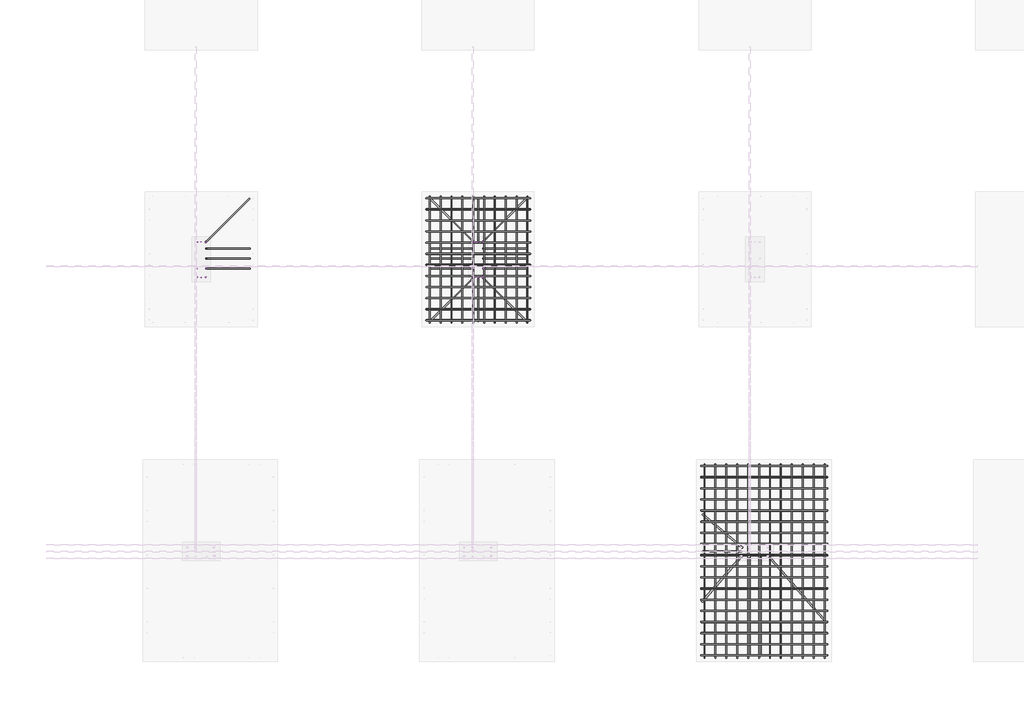
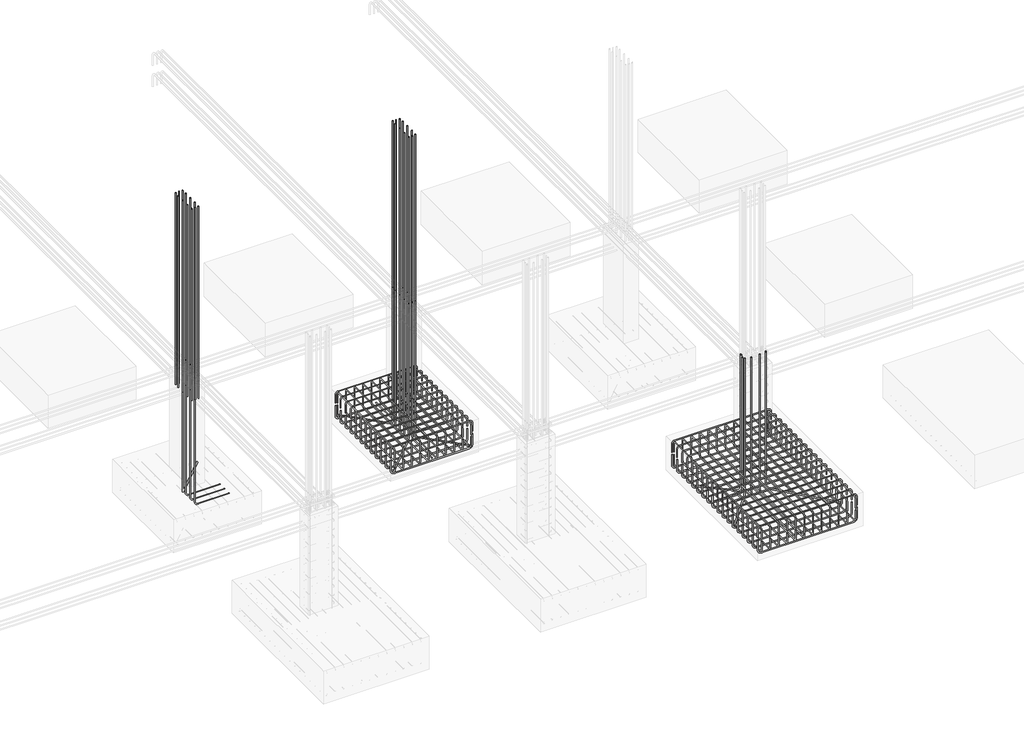
# One storey, part 6 of 18: 39 reinforcing bars.
"""IFC4 building model written with IfcOpenShell, lengths in millimetres."""

from ifc_helpers import new_model, si_unit, point, frame, origin, place, context, project, spatial, polyline, circle_curve, trimmed, segment, composite_curve, source, transform, mapped, element, save
from ifc_brep_helpers import swept_disk

model = new_model("IFC4")

# Units and contexts
model_context = context("Model", 3, world=origin())
ifc_project = project(units=[si_unit("LENGTHUNIT", "METRE", prefix="MILLI")], contexts=[model_context])

# Site, building, storey
site = spatial("IfcSite", under=ifc_project)
building = spatial("IfcBuilding", under=site)
storey = spatial("IfcBuildingStorey", under=building, Elevation=-2000.0)

# Reinforcing bars
placement = place(None, origin())
reinforcing_bar_shape = source(origin(), model_context, "Body", "SolidModel", [
    swept_disk(composite_curve([segment(polyline([(-778.5399692, -834.8555128, -2300.0), (-778.5399692, -834.8555128, -2486.6)]), True, "CONTINUOUS"), segment(trimmed(circle_curve(frame((-833.9899692, -834.8555128, -2486.6), z_axis=(0.0, 1.0, 0.0), x_axis=(55.450000000000045, 0.0, 0.0)), 55.45), [point((-778.5399692, -834.8555128, -2486.6))], [point((-833.9899692, -834.8555128, -2542.05))], True, "CARTESIAN"), True, "CONTINUOUS"), segment(polyline([(-833.9899692, -834.8555128, -2542.05), (-2107.1899692, -834.8555128, -2542.05)]), True, "CONTINUOUS"), segment(trimmed(circle_curve(frame((-2107.1899692, -834.8555128, -2486.6), z_axis=(0.0, 1.0, 0.0), x_axis=(0.0, 0.0, -55.45000000000027)), 55.45), [point((-2107.1899692, -834.8555128, -2542.05))], [point((-2162.6399692, -834.8555128, -2486.6))], True, "CARTESIAN"), True, "CONTINUOUS"), segment(polyline([(-2162.6399692, -834.8555128, -2486.6), (-2162.6399692, -834.8555128, -2300.0)]), True, "CONTINUOUS")], self_intersect=False), 7.95),
])
element("IfcReinforcingBar", 1, at=placement, inside=storey, context=model_context, shape_type="MappedRepresentation", body=[
    mapped(reinforcing_bar_shape, transform((0.0, 0.0, 0.0), x_axis=(1.0, 0.0, 0.0), y_axis=(0.0, 1.0, 0.0), z_axis=(0.0, 0.0, 1.0))),
    mapped(reinforcing_bar_shape, transform((0.0, -148.4250709, 0.0), x_axis=(1.0, 0.0, 0.0), y_axis=(0.0, 1.0, 0.0), z_axis=(0.0, 0.0, 1.0))),
    mapped(reinforcing_bar_shape, transform((0.0, -296.8501418, 0.0), x_axis=(1.0, 0.0, 0.0), y_axis=(0.0, 1.0, 0.0), z_axis=(0.0, 0.0, 1.0))),
    mapped(reinforcing_bar_shape, transform((0.0, -445.2752126, 0.0), x_axis=(1.0, 0.0, 0.0), y_axis=(0.0, 1.0, 0.0), z_axis=(0.0, 0.0, 1.0))),
    mapped(reinforcing_bar_shape, transform((0.0, -593.7002835, 0.0), x_axis=(1.0, 0.0, 0.0), y_axis=(0.0, 1.0, 0.0), z_axis=(0.0, 0.0, 1.0))),
    mapped(reinforcing_bar_shape, transform((0.0, -742.1253544, 0.0), x_axis=(1.0, 0.0, 0.0), y_axis=(0.0, 1.0, 0.0), z_axis=(0.0, 0.0, 1.0))),
    mapped(reinforcing_bar_shape, transform((0.0, -890.5504253, 0.0), x_axis=(1.0, 0.0, 0.0), y_axis=(0.0, 1.0, 0.0), z_axis=(0.0, 0.0, 1.0))),
    mapped(reinforcing_bar_shape, transform((0.0, -1038.9754961, 0.0), x_axis=(1.0, 0.0, 0.0), y_axis=(0.0, 1.0, 0.0), z_axis=(0.0, 0.0, 1.0))),
    mapped(reinforcing_bar_shape, transform((0.0, -1187.400567, 0.0), x_axis=(1.0, 0.0, 0.0), y_axis=(0.0, 1.0, 0.0), z_axis=(0.0, 0.0, 1.0))),
    mapped(reinforcing_bar_shape, transform((0.0, -1335.8256379, 0.0), x_axis=(1.0, 0.0, 0.0), y_axis=(0.0, 1.0, 0.0), z_axis=(0.0, 0.0, 1.0))),
    mapped(reinforcing_bar_shape, transform((0.0, -1484.2507088, 0.0), x_axis=(1.0, 0.0, 0.0), y_axis=(0.0, 1.0, 0.0), z_axis=(0.0, 0.0, 1.0))),
    mapped(reinforcing_bar_shape, transform((0.0, -1632.6757796, 0.0), x_axis=(1.0, 0.0, 0.0), y_axis=(0.0, 1.0, 0.0), z_axis=(0.0, 0.0, 1.0))),
])
reinforcing_bar_2_shape = source(origin(), model_context, "Body", "SolidModel", [
    swept_disk(composite_curve([segment(polyline([(-2164.5899692, -834.8555128, -2250.0), (-2164.5899692, -834.8555128, -2102.0)]), True, "CONTINUOUS"), segment(trimmed(circle_curve(frame((-2118.5899692, -834.8555128, -2102.0), z_axis=(0.0, 1.0, 0.0), x_axis=(-46.0, 0.0, 0.0)), 46.0), [point((-2164.5899692, -834.8555128, -2102.0))], [point((-2118.5899692, -834.8555128, -2056.0))], True, "CARTESIAN"), True, "CONTINUOUS"), segment(polyline([(-2118.5899692, -834.8555128, -2056.0), (-822.5899692, -834.8555128, -2056.0)]), True, "CONTINUOUS"), segment(trimmed(circle_curve(frame((-822.5899692, -834.8555128, -2102.0), z_axis=(0.0, 1.0, 0.0), x_axis=(0.0, 0.0, 46.0)), 46.0), [point((-822.5899692, -834.8555128, -2056.0))], [point((-776.5899692, -834.8555128, -2102.0))], True, "CARTESIAN"), True, "CONTINUOUS"), segment(polyline([(-776.5899692, -834.8555128, -2102.0), (-776.5899692, -834.8555128, -2250.0)]), True, "CONTINUOUS")], self_intersect=False), 6.0),
])
element("IfcReinforcingBar", 2, at=placement, inside=storey, context=model_context, shape_type="MappedRepresentation", body=[
    mapped(reinforcing_bar_2_shape, transform((0.0, 0.0, 0.0), x_axis=(1.0, 0.0, 0.0), y_axis=(0.0, 1.0, 0.0), z_axis=(0.0, 0.0, 1.0))),
    mapped(reinforcing_bar_2_shape, transform((0.0, -148.4250709, 0.0), x_axis=(1.0, 0.0, 0.0), y_axis=(0.0, 1.0, 0.0), z_axis=(0.0, 0.0, 1.0))),
    mapped(reinforcing_bar_2_shape, transform((0.0, -296.8501418, 0.0), x_axis=(1.0, 0.0, 0.0), y_axis=(0.0, 1.0, 0.0), z_axis=(0.0, 0.0, 1.0))),
    mapped(reinforcing_bar_2_shape, transform((0.0, -445.2752126, 0.0), x_axis=(1.0, 0.0, 0.0), y_axis=(0.0, 1.0, 0.0), z_axis=(0.0, 0.0, 1.0))),
    mapped(reinforcing_bar_2_shape, transform((0.0, -593.7002835, 0.0), x_axis=(1.0, 0.0, 0.0), y_axis=(0.0, 1.0, 0.0), z_axis=(0.0, 0.0, 1.0))),
    mapped(reinforcing_bar_2_shape, transform((0.0, -742.1253544, 0.0), x_axis=(1.0, 0.0, 0.0), y_axis=(0.0, 1.0, 0.0), z_axis=(0.0, 0.0, 1.0))),
    mapped(reinforcing_bar_2_shape, transform((0.0, -890.5504253, 0.0), x_axis=(1.0, 0.0, 0.0), y_axis=(0.0, 1.0, 0.0), z_axis=(0.0, 0.0, 1.0))),
    mapped(reinforcing_bar_2_shape, transform((0.0, -1038.9754961, 0.0), x_axis=(1.0, 0.0, 0.0), y_axis=(0.0, 1.0, 0.0), z_axis=(0.0, 0.0, 1.0))),
    mapped(reinforcing_bar_2_shape, transform((0.0, -1187.400567, 0.0), x_axis=(1.0, 0.0, 0.0), y_axis=(0.0, 1.0, 0.0), z_axis=(0.0, 0.0, 1.0))),
    mapped(reinforcing_bar_2_shape, transform((0.0, -1335.8256379, 0.0), x_axis=(1.0, 0.0, 0.0), y_axis=(0.0, 1.0, 0.0), z_axis=(0.0, 0.0, 1.0))),
    mapped(reinforcing_bar_2_shape, transform((0.0, -1484.2507088, 0.0), x_axis=(1.0, 0.0, 0.0), y_axis=(0.0, 1.0, 0.0), z_axis=(0.0, 0.0, 1.0))),
    mapped(reinforcing_bar_2_shape, transform((0.0, -1632.6757796, 0.0), x_axis=(1.0, 0.0, 0.0), y_axis=(0.0, 1.0, 0.0), z_axis=(0.0, 0.0, 1.0))),
])
reinforcing_bar_3_shape = source(origin(), model_context, "Body", "SolidModel", [
    swept_disk(composite_curve([segment(polyline([(-2118.4091864, -811.9600376, -2322.6684255), (-2118.4091864, -811.9600376, -2470.6684255)]), True, "CONTINUOUS"), segment(trimmed(circle_curve(frame((-2118.4091864, -857.9600376, -2470.6684255), z_axis=(-1.0, 0.0, 0.0), x_axis=(0.0, 46.0, 0.0)), 46.0), [point((-2118.4091864, -811.9600376, -2470.6684255))], [point((-2118.4091864, -857.9600376, -2516.6684255))], True, "CARTESIAN"), True, "CONTINUOUS"), segment(polyline([(-2118.4091864, -857.9600376, -2516.6684255), (-2118.4091864, -2453.9600376, -2516.6684255)]), True, "CONTINUOUS"), segment(trimmed(circle_curve(frame((-2118.4091864, -2453.9600376, -2470.6684255), z_axis=(-1.0, 0.0, 0.0), x_axis=(0.0, 0.0, -46.0)), 46.0), [point((-2118.4091864, -2453.9600376, -2516.6684255))], [point((-2118.4091864, -2499.9600376, -2470.6684255))], True, "CARTESIAN"), True, "CONTINUOUS"), segment(polyline([(-2118.4091864, -2499.9600376, -2470.6684255), (-2118.4091864, -2499.9600376, -2322.6684255)]), True, "CONTINUOUS")], self_intersect=False), 6.0),
])
element("IfcReinforcingBar", 3, at=placement, inside=storey, context=model_context, shape_type="MappedRepresentation", body=[
    mapped(reinforcing_bar_3_shape, transform((0.0, 0.0, 0.0), x_axis=(1.0, 0.0, 0.0), y_axis=(0.0, 1.0, 0.0), z_axis=(0.0, 0.0, 1.0))),
    mapped(reinforcing_bar_3_shape, transform((144.8687847, 0.0, 0.0), x_axis=(1.0, 0.0, 0.0), y_axis=(0.0, 1.0, 0.0), z_axis=(0.0, 0.0, 1.0))),
    mapped(reinforcing_bar_3_shape, transform((289.7375694, 0.0, 0.0), x_axis=(1.0, 0.0, 0.0), y_axis=(0.0, 1.0, 0.0), z_axis=(0.0, 0.0, 1.0))),
    mapped(reinforcing_bar_3_shape, transform((434.6063541, 0.0, 0.0), x_axis=(1.0, 0.0, 0.0), y_axis=(0.0, 1.0, 0.0), z_axis=(0.0, 0.0, 1.0))),
    mapped(reinforcing_bar_3_shape, transform((579.4751388, 0.0, 0.0), x_axis=(1.0, 0.0, 0.0), y_axis=(0.0, 1.0, 0.0), z_axis=(0.0, 0.0, 1.0))),
    mapped(reinforcing_bar_3_shape, transform((724.3439235, 0.0, 0.0), x_axis=(1.0, 0.0, 0.0), y_axis=(0.0, 1.0, 0.0), z_axis=(0.0, 0.0, 1.0))),
    mapped(reinforcing_bar_3_shape, transform((869.2127082, 0.0, 0.0), x_axis=(1.0, 0.0, 0.0), y_axis=(0.0, 1.0, 0.0), z_axis=(0.0, 0.0, 1.0))),
    mapped(reinforcing_bar_3_shape, transform((1014.0814929, 0.0, 0.0), x_axis=(1.0, 0.0, 0.0), y_axis=(0.0, 1.0, 0.0), z_axis=(0.0, 0.0, 1.0))),
    mapped(reinforcing_bar_3_shape, transform((1158.9502776, 0.0, 0.0), x_axis=(1.0, 0.0, 0.0), y_axis=(0.0, 1.0, 0.0), z_axis=(0.0, 0.0, 1.0))),
    mapped(reinforcing_bar_3_shape, transform((1303.8190623, 0.0, 0.0), x_axis=(1.0, 0.0, 0.0), y_axis=(0.0, 1.0, 0.0), z_axis=(0.0, 0.0, 1.0))),
])
reinforcing_bar_4_shape = source(origin(), model_context, "Body", "SolidModel", [
    swept_disk(composite_curve([segment(polyline([(-812.6669522, -811.9600376, -2276.6677805), (-812.6669522, -811.9600376, -2128.6677805)]), True, "CONTINUOUS"), segment(trimmed(circle_curve(frame((-812.6669522, -857.9600376, -2128.6677805), z_axis=(1.0, 0.0, 0.0), x_axis=(0.0, 46.0, 0.0)), 46.0), [point((-812.6669522, -811.9600376, -2128.6677805))], [point((-812.6669522, -857.9600376, -2082.6677805))], True, "CARTESIAN"), True, "CONTINUOUS"), segment(polyline([(-812.6669522, -857.9600376, -2082.6677805), (-812.6669522, -2453.9600376, -2082.6677805)]), True, "CONTINUOUS"), segment(trimmed(circle_curve(frame((-812.6669522, -2453.9600376, -2128.6677805), z_axis=(1.0, 0.0, 0.0), x_axis=(0.0, 0.0, 46.0)), 46.0), [point((-812.6669522, -2453.9600376, -2082.6677805))], [point((-812.6669522, -2499.9600376, -2128.6677805))], True, "CARTESIAN"), True, "CONTINUOUS"), segment(polyline([(-812.6669522, -2499.9600376, -2128.6677805), (-812.6669522, -2499.9600376, -2276.6677805)]), True, "CONTINUOUS")], self_intersect=False), 6.0),
])
element("IfcReinforcingBar", 4, at=placement, inside=storey, context=model_context, shape_type="MappedRepresentation", body=[
    mapped(reinforcing_bar_4_shape, transform((0.0, 0.0, 0.0), x_axis=(1.0, 0.0, 0.0), y_axis=(0.0, 1.0, 0.0), z_axis=(0.0, 0.0, 1.0))),
    mapped(reinforcing_bar_4_shape, transform((-145.0824705, 0.0, 0.0), x_axis=(1.0, 0.0, 0.0), y_axis=(0.0, 1.0, 0.0), z_axis=(0.0, 0.0, 1.0))),
    mapped(reinforcing_bar_4_shape, transform((-290.1649409, 0.0, 0.0), x_axis=(1.0, 0.0, 0.0), y_axis=(0.0, 1.0, 0.0), z_axis=(0.0, 0.0, 1.0))),
    mapped(reinforcing_bar_4_shape, transform((-435.2474114, 0.0, 0.0), x_axis=(1.0, 0.0, 0.0), y_axis=(0.0, 1.0, 0.0), z_axis=(0.0, 0.0, 1.0))),
    mapped(reinforcing_bar_4_shape, transform((-580.3298819, 0.0, 0.0), x_axis=(1.0, 0.0, 0.0), y_axis=(0.0, 1.0, 0.0), z_axis=(0.0, 0.0, 1.0))),
    mapped(reinforcing_bar_4_shape, transform((-725.4123523, 0.0, 0.0), x_axis=(1.0, 0.0, 0.0), y_axis=(0.0, 1.0, 0.0), z_axis=(0.0, 0.0, 1.0))),
    mapped(reinforcing_bar_4_shape, transform((-870.4948228, 0.0, 0.0), x_axis=(1.0, 0.0, 0.0), y_axis=(0.0, 1.0, 0.0), z_axis=(0.0, 0.0, 1.0))),
    mapped(reinforcing_bar_4_shape, transform((-1015.5772932, 0.0, 0.0), x_axis=(1.0, 0.0, 0.0), y_axis=(0.0, 1.0, 0.0), z_axis=(0.0, 0.0, 1.0))),
    mapped(reinforcing_bar_4_shape, transform((-1160.6597637, 0.0, 0.0), x_axis=(1.0, 0.0, 0.0), y_axis=(0.0, 1.0, 0.0), z_axis=(0.0, 0.0, 1.0))),
    mapped(reinforcing_bar_4_shape, transform((-1305.7422342, 0.0, 0.0), x_axis=(1.0, 0.0, 0.0), y_axis=(0.0, 1.0, 0.0), z_axis=(0.0, 0.0, 1.0))),
])
reinforcing_bar_5_shape = source(origin(), model_context, "Body", "SolidModel", [
    swept_disk(composite_curve([segment(polyline([(3191.7059943, -4415.5752408, -2300.0), (3191.7059943, -4415.5752408, -2486.6)]), True, "CONTINUOUS"), segment(trimmed(circle_curve(frame((3136.2559943, -4415.5752408, -2486.6), z_axis=(0.0, 1.0, 0.0), x_axis=(55.44999999999982, 0.0, 0.0)), 55.45), [point((3191.7059943, -4415.5752408, -2486.6))], [point((3136.2559943, -4415.5752408, -2542.05))], True, "CARTESIAN"), True, "CONTINUOUS"), segment(polyline([(3136.2559943, -4415.5752408, -2542.05), (1563.0559943, -4415.5752408, -2542.05)]), True, "CONTINUOUS"), segment(trimmed(circle_curve(frame((1563.0559943, -4415.5752408, -2486.6), z_axis=(0.0, 1.0, 0.0), x_axis=(0.0, 0.0, -55.45000000000027)), 55.45), [point((1563.0559943, -4415.5752408, -2542.05))], [point((1507.6059943, -4415.5752408, -2486.6))], True, "CARTESIAN"), True, "CONTINUOUS"), segment(polyline([(1507.6059943, -4415.5752408, -2486.6), (1507.6059943, -4415.5752408, -2300.0)]), True, "CONTINUOUS")], self_intersect=False), 7.95),
])
element("IfcReinforcingBar", 5, at=placement, inside=storey, context=model_context, shape_type="MappedRepresentation", body=[
    mapped(reinforcing_bar_5_shape, transform((0.0, 0.0, 0.0), x_axis=(1.0, 0.0, 0.0), y_axis=(0.0, 1.0, 0.0), z_axis=(0.0, 0.0, 1.0))),
    mapped(reinforcing_bar_5_shape, transform((0.0, -148.9809282, 0.0), x_axis=(1.0, 0.0, 0.0), y_axis=(0.0, 1.0, 0.0), z_axis=(0.0, 0.0, 1.0))),
    mapped(reinforcing_bar_5_shape, transform((0.0, -297.9618564, 0.0), x_axis=(1.0, 0.0, 0.0), y_axis=(0.0, 1.0, 0.0), z_axis=(0.0, 0.0, 1.0))),
    mapped(reinforcing_bar_5_shape, transform((0.0, -446.9427846, 0.0), x_axis=(1.0, 0.0, 0.0), y_axis=(0.0, 1.0, 0.0), z_axis=(0.0, 0.0, 1.0))),
    mapped(reinforcing_bar_5_shape, transform((0.0, -595.9237129, 0.0), x_axis=(1.0, 0.0, 0.0), y_axis=(0.0, 1.0, 0.0), z_axis=(0.0, 0.0, 1.0))),
    mapped(reinforcing_bar_5_shape, transform((0.0, -744.9046411, 0.0), x_axis=(1.0, 0.0, 0.0), y_axis=(0.0, 1.0, 0.0), z_axis=(0.0, 0.0, 1.0))),
    mapped(reinforcing_bar_5_shape, transform((0.0, -893.8855693, 0.0), x_axis=(1.0, 0.0, 0.0), y_axis=(0.0, 1.0, 0.0), z_axis=(0.0, 0.0, 1.0))),
    mapped(reinforcing_bar_5_shape, transform((0.0, -1042.8664975, 0.0), x_axis=(1.0, 0.0, 0.0), y_axis=(0.0, 1.0, 0.0), z_axis=(0.0, 0.0, 1.0))),
    mapped(reinforcing_bar_5_shape, transform((0.0, -1191.8474257, 0.0), x_axis=(1.0, 0.0, 0.0), y_axis=(0.0, 1.0, 0.0), z_axis=(0.0, 0.0, 1.0))),
    mapped(reinforcing_bar_5_shape, transform((0.0, -1340.8283539, 0.0), x_axis=(1.0, 0.0, 0.0), y_axis=(0.0, 1.0, 0.0), z_axis=(0.0, 0.0, 1.0))),
    mapped(reinforcing_bar_5_shape, transform((0.0, -1489.8092821, 0.0), x_axis=(1.0, 0.0, 0.0), y_axis=(0.0, 1.0, 0.0), z_axis=(0.0, 0.0, 1.0))),
    mapped(reinforcing_bar_5_shape, transform((0.0, -1638.7902103, 0.0), x_axis=(1.0, 0.0, 0.0), y_axis=(0.0, 1.0, 0.0), z_axis=(0.0, 0.0, 1.0))),
    mapped(reinforcing_bar_5_shape, transform((0.0, -1787.7711386, 0.0), x_axis=(1.0, 0.0, 0.0), y_axis=(0.0, 1.0, 0.0), z_axis=(0.0, 0.0, 1.0))),
    mapped(reinforcing_bar_5_shape, transform((0.0, -1936.7520668, 0.0), x_axis=(1.0, 0.0, 0.0), y_axis=(0.0, 1.0, 0.0), z_axis=(0.0, 0.0, 1.0))),
    mapped(reinforcing_bar_5_shape, transform((0.0, -2085.732995, 0.0), x_axis=(1.0, 0.0, 0.0), y_axis=(0.0, 1.0, 0.0), z_axis=(0.0, 0.0, 1.0))),
    mapped(reinforcing_bar_5_shape, transform((0.0, -2234.7139232, 0.0), x_axis=(1.0, 0.0, 0.0), y_axis=(0.0, 1.0, 0.0), z_axis=(0.0, 0.0, 1.0))),
    mapped(reinforcing_bar_5_shape, transform((0.0, -2383.6948514, 0.0), x_axis=(1.0, 0.0, 0.0), y_axis=(0.0, 1.0, 0.0), z_axis=(0.0, 0.0, 1.0))),
    mapped(reinforcing_bar_5_shape, transform((0.0, -2532.6757796, 0.0), x_axis=(1.0, 0.0, 0.0), y_axis=(0.0, 1.0, 0.0), z_axis=(0.0, 0.0, 1.0))),
])
reinforcing_bar_6_shape = source(origin(), model_context, "Body", "SolidModel", [
    swept_disk(composite_curve([segment(polyline([(1505.6559943, -4415.5752408, -2250.0), (1505.6559943, -4415.5752408, -2102.0)]), True, "CONTINUOUS"), segment(trimmed(circle_curve(frame((1551.6559943, -4415.5752408, -2102.0), z_axis=(0.0, 1.0, 0.0), x_axis=(-46.0, 0.0, 0.0)), 46.0), [point((1505.6559943, -4415.5752408, -2102.0))], [point((1551.6559943, -4415.5752408, -2056.0))], True, "CARTESIAN"), True, "CONTINUOUS"), segment(polyline([(1551.6559943, -4415.5752408, -2056.0), (3147.6559943, -4415.5752408, -2056.0)]), True, "CONTINUOUS"), segment(trimmed(circle_curve(frame((3147.6559943, -4415.5752408, -2102.0), z_axis=(0.0, 1.0, 0.0), x_axis=(0.0, 0.0, 46.0)), 46.0), [point((3147.6559943, -4415.5752408, -2056.0))], [point((3193.6559943, -4415.5752408, -2102.0))], True, "CARTESIAN"), True, "CONTINUOUS"), segment(polyline([(3193.6559943, -4415.5752408, -2102.0), (3193.6559943, -4415.5752408, -2250.0)]), True, "CONTINUOUS")], self_intersect=False), 6.0),
])
element("IfcReinforcingBar", 6, at=placement, inside=storey, context=model_context, shape_type="MappedRepresentation", body=[
    mapped(reinforcing_bar_6_shape, transform((0.0, 0.0, 0.0), x_axis=(1.0, 0.0, 0.0), y_axis=(0.0, 1.0, 0.0), z_axis=(0.0, 0.0, 1.0))),
    mapped(reinforcing_bar_6_shape, transform((0.0, -148.9809282, 0.0), x_axis=(1.0, 0.0, 0.0), y_axis=(0.0, 1.0, 0.0), z_axis=(0.0, 0.0, 1.0))),
    mapped(reinforcing_bar_6_shape, transform((0.0, -297.9618564, 0.0), x_axis=(1.0, 0.0, 0.0), y_axis=(0.0, 1.0, 0.0), z_axis=(0.0, 0.0, 1.0))),
    mapped(reinforcing_bar_6_shape, transform((0.0, -446.9427846, 0.0), x_axis=(1.0, 0.0, 0.0), y_axis=(0.0, 1.0, 0.0), z_axis=(0.0, 0.0, 1.0))),
    mapped(reinforcing_bar_6_shape, transform((0.0, -595.9237129, 0.0), x_axis=(1.0, 0.0, 0.0), y_axis=(0.0, 1.0, 0.0), z_axis=(0.0, 0.0, 1.0))),
    mapped(reinforcing_bar_6_shape, transform((0.0, -744.9046411, 0.0), x_axis=(1.0, 0.0, 0.0), y_axis=(0.0, 1.0, 0.0), z_axis=(0.0, 0.0, 1.0))),
    mapped(reinforcing_bar_6_shape, transform((0.0, -893.8855693, 0.0), x_axis=(1.0, 0.0, 0.0), y_axis=(0.0, 1.0, 0.0), z_axis=(0.0, 0.0, 1.0))),
    mapped(reinforcing_bar_6_shape, transform((0.0, -1042.8664975, 0.0), x_axis=(1.0, 0.0, 0.0), y_axis=(0.0, 1.0, 0.0), z_axis=(0.0, 0.0, 1.0))),
    mapped(reinforcing_bar_6_shape, transform((0.0, -1191.8474257, 0.0), x_axis=(1.0, 0.0, 0.0), y_axis=(0.0, 1.0, 0.0), z_axis=(0.0, 0.0, 1.0))),
    mapped(reinforcing_bar_6_shape, transform((0.0, -1340.8283539, 0.0), x_axis=(1.0, 0.0, 0.0), y_axis=(0.0, 1.0, 0.0), z_axis=(0.0, 0.0, 1.0))),
    mapped(reinforcing_bar_6_shape, transform((0.0, -1489.8092821, 0.0), x_axis=(1.0, 0.0, 0.0), y_axis=(0.0, 1.0, 0.0), z_axis=(0.0, 0.0, 1.0))),
    mapped(reinforcing_bar_6_shape, transform((0.0, -1638.7902103, 0.0), x_axis=(1.0, 0.0, 0.0), y_axis=(0.0, 1.0, 0.0), z_axis=(0.0, 0.0, 1.0))),
    mapped(reinforcing_bar_6_shape, transform((0.0, -1787.7711386, 0.0), x_axis=(1.0, 0.0, 0.0), y_axis=(0.0, 1.0, 0.0), z_axis=(0.0, 0.0, 1.0))),
    mapped(reinforcing_bar_6_shape, transform((0.0, -1936.7520668, 0.0), x_axis=(1.0, 0.0, 0.0), y_axis=(0.0, 1.0, 0.0), z_axis=(0.0, 0.0, 1.0))),
    mapped(reinforcing_bar_6_shape, transform((0.0, -2085.732995, 0.0), x_axis=(1.0, 0.0, 0.0), y_axis=(0.0, 1.0, 0.0), z_axis=(0.0, 0.0, 1.0))),
    mapped(reinforcing_bar_6_shape, transform((0.0, -2234.7139232, 0.0), x_axis=(1.0, 0.0, 0.0), y_axis=(0.0, 1.0, 0.0), z_axis=(0.0, 0.0, 1.0))),
    mapped(reinforcing_bar_6_shape, transform((0.0, -2383.6948514, 0.0), x_axis=(1.0, 0.0, 0.0), y_axis=(0.0, 1.0, 0.0), z_axis=(0.0, 0.0, 1.0))),
    mapped(reinforcing_bar_6_shape, transform((0.0, -2532.6757796, 0.0), x_axis=(1.0, 0.0, 0.0), y_axis=(0.0, 1.0, 0.0), z_axis=(0.0, 0.0, 1.0))),
])
reinforcing_bar_7_shape = source(origin(), model_context, "Body", "SolidModel", [
    swept_disk(composite_curve([segment(polyline([(1551.8367771, -4392.6797656, -2322.6684255), (1551.8367771, -4392.6797656, -2470.6684255)]), True, "CONTINUOUS"), segment(trimmed(circle_curve(frame((1551.8367771, -4438.6797656, -2470.6684255), z_axis=(-1.0, 0.0, 0.0), x_axis=(0.0, 46.0, 0.0)), 46.0), [point((1551.8367771, -4392.6797656, -2470.6684255))], [point((1551.8367771, -4438.6797656, -2516.6684255))], True, "CARTESIAN"), True, "CONTINUOUS"), segment(polyline([(1551.8367771, -4438.6797656, -2516.6684255), (1551.8367771, -6934.6797656, -2516.6684255)]), True, "CONTINUOUS"), segment(trimmed(circle_curve(frame((1551.8367771, -6934.6797656, -2470.6684255), z_axis=(-1.0, 0.0, 0.0), x_axis=(0.0, 0.0, -46.0)), 46.0), [point((1551.8367771, -6934.6797656, -2516.6684255))], [point((1551.8367771, -6980.6797656, -2470.6684255))], True, "CARTESIAN"), True, "CONTINUOUS"), segment(polyline([(1551.8367771, -6980.6797656, -2470.6684255), (1551.8367771, -6980.6797656, -2322.6684255)]), True, "CONTINUOUS")], self_intersect=False), 6.0),
])
element("IfcReinforcingBar", 7, at=placement, inside=storey, context=model_context, shape_type="MappedRepresentation", body=[
    mapped(reinforcing_bar_7_shape, transform((0.0, 0.0, 0.0), x_axis=(1.0, 0.0, 0.0), y_axis=(0.0, 1.0, 0.0), z_axis=(0.0, 0.0, 1.0))),
    mapped(reinforcing_bar_7_shape, transform((145.8017329, 0.0, 0.0), x_axis=(1.0, 0.0, 0.0), y_axis=(0.0, 1.0, 0.0), z_axis=(0.0, 0.0, 1.0))),
    mapped(reinforcing_bar_7_shape, transform((291.6034659, 0.0, 0.0), x_axis=(1.0, 0.0, 0.0), y_axis=(0.0, 1.0, 0.0), z_axis=(0.0, 0.0, 1.0))),
    mapped(reinforcing_bar_7_shape, transform((437.4051988, 0.0, 0.0), x_axis=(1.0, 0.0, 0.0), y_axis=(0.0, 1.0, 0.0), z_axis=(0.0, 0.0, 1.0))),
    mapped(reinforcing_bar_7_shape, transform((583.2069318, 0.0, 0.0), x_axis=(1.0, 0.0, 0.0), y_axis=(0.0, 1.0, 0.0), z_axis=(0.0, 0.0, 1.0))),
    mapped(reinforcing_bar_7_shape, transform((729.0086647, 0.0, 0.0), x_axis=(1.0, 0.0, 0.0), y_axis=(0.0, 1.0, 0.0), z_axis=(0.0, 0.0, 1.0))),
    mapped(reinforcing_bar_7_shape, transform((874.8103976, 0.0, 0.0), x_axis=(1.0, 0.0, 0.0), y_axis=(0.0, 1.0, 0.0), z_axis=(0.0, 0.0, 1.0))),
    mapped(reinforcing_bar_7_shape, transform((1020.6121306, 0.0, 0.0), x_axis=(1.0, 0.0, 0.0), y_axis=(0.0, 1.0, 0.0), z_axis=(0.0, 0.0, 1.0))),
    mapped(reinforcing_bar_7_shape, transform((1166.4138635, 0.0, 0.0), x_axis=(1.0, 0.0, 0.0), y_axis=(0.0, 1.0, 0.0), z_axis=(0.0, 0.0, 1.0))),
    mapped(reinforcing_bar_7_shape, transform((1312.2155965, 0.0, 0.0), x_axis=(1.0, 0.0, 0.0), y_axis=(0.0, 1.0, 0.0), z_axis=(0.0, 0.0, 1.0))),
    mapped(reinforcing_bar_7_shape, transform((1458.0173294, 0.0, 0.0), x_axis=(1.0, 0.0, 0.0), y_axis=(0.0, 1.0, 0.0), z_axis=(0.0, 0.0, 1.0))),
    mapped(reinforcing_bar_7_shape, transform((1603.8190623, 0.0, 0.0), x_axis=(1.0, 0.0, 0.0), y_axis=(0.0, 1.0, 0.0), z_axis=(0.0, 0.0, 1.0))),
])
reinforcing_bar_8_shape = source(origin(), model_context, "Body", "SolidModel", [
    swept_disk(composite_curve([segment(polyline([(3157.5790113, -4392.6797656, -2276.6677805), (3157.5790113, -4392.6797656, -2128.6677805)]), True, "CONTINUOUS"), segment(trimmed(circle_curve(frame((3157.5790113, -4438.6797656, -2128.6677805), z_axis=(1.0, 0.0, 0.0), x_axis=(0.0, 46.0, 0.0)), 46.0), [point((3157.5790113, -4392.6797656, -2128.6677805))], [point((3157.5790113, -4438.6797656, -2082.6677805))], True, "CARTESIAN"), True, "CONTINUOUS"), segment(polyline([(3157.5790113, -4438.6797656, -2082.6677805), (3157.5790113, -6934.6797656, -2082.6677805)]), True, "CONTINUOUS"), segment(trimmed(circle_curve(frame((3157.5790113, -6934.6797656, -2128.6677805), z_axis=(1.0, 0.0, 0.0), x_axis=(0.0, 0.0, 46.0)), 46.0), [point((3157.5790113, -6934.6797656, -2082.6677805))], [point((3157.5790113, -6980.6797656, -2128.6677805))], True, "CARTESIAN"), True, "CONTINUOUS"), segment(polyline([(3157.5790113, -6980.6797656, -2128.6677805), (3157.5790113, -6980.6797656, -2276.6677805)]), True, "CONTINUOUS")], self_intersect=False), 6.0),
])
element("IfcReinforcingBar", 8, at=placement, inside=storey, context=model_context, shape_type="MappedRepresentation", body=[
    mapped(reinforcing_bar_8_shape, transform((0.0, 0.0, 0.0), x_axis=(1.0, 0.0, 0.0), y_axis=(0.0, 1.0, 0.0), z_axis=(0.0, 0.0, 1.0))),
    mapped(reinforcing_bar_8_shape, transform((-145.9765667, 0.0, 0.0), x_axis=(1.0, 0.0, 0.0), y_axis=(0.0, 1.0, 0.0), z_axis=(0.0, 0.0, 1.0))),
    mapped(reinforcing_bar_8_shape, transform((-291.9531335, 0.0, 0.0), x_axis=(1.0, 0.0, 0.0), y_axis=(0.0, 1.0, 0.0), z_axis=(0.0, 0.0, 1.0))),
    mapped(reinforcing_bar_8_shape, transform((-437.9297002, 0.0, 0.0), x_axis=(1.0, 0.0, 0.0), y_axis=(0.0, 1.0, 0.0), z_axis=(0.0, 0.0, 1.0))),
    mapped(reinforcing_bar_8_shape, transform((-583.906267, 0.0, 0.0), x_axis=(1.0, 0.0, 0.0), y_axis=(0.0, 1.0, 0.0), z_axis=(0.0, 0.0, 1.0))),
    mapped(reinforcing_bar_8_shape, transform((-729.8828337, 0.0, 0.0), x_axis=(1.0, 0.0, 0.0), y_axis=(0.0, 1.0, 0.0), z_axis=(0.0, 0.0, 1.0))),
    mapped(reinforcing_bar_8_shape, transform((-875.8594005, 0.0, 0.0), x_axis=(1.0, 0.0, 0.0), y_axis=(0.0, 1.0, 0.0), z_axis=(0.0, 0.0, 1.0))),
    mapped(reinforcing_bar_8_shape, transform((-1021.8359672, 0.0, 0.0), x_axis=(1.0, 0.0, 0.0), y_axis=(0.0, 1.0, 0.0), z_axis=(0.0, 0.0, 1.0))),
    mapped(reinforcing_bar_8_shape, transform((-1167.8125339, 0.0, 0.0), x_axis=(1.0, 0.0, 0.0), y_axis=(0.0, 1.0, 0.0), z_axis=(0.0, 0.0, 1.0))),
    mapped(reinforcing_bar_8_shape, transform((-1313.7891007, 0.0, 0.0), x_axis=(1.0, 0.0, 0.0), y_axis=(0.0, 1.0, 0.0), z_axis=(0.0, 0.0, 1.0))),
    mapped(reinforcing_bar_8_shape, transform((-1459.7656674, 0.0, 0.0), x_axis=(1.0, 0.0, 0.0), y_axis=(0.0, 1.0, 0.0), z_axis=(0.0, 0.0, 1.0))),
    mapped(reinforcing_bar_8_shape, transform((-1605.7422342, 0.0, 0.0), x_axis=(1.0, 0.0, 0.0), y_axis=(0.0, 1.0, 0.0), z_axis=(0.0, 0.0, 1.0))),
])
element("IfcReinforcingBar", 9, at=placement, inside=storey, context=model_context, shape_type="SolidModel", body=[
    swept_disk(composite_curve([segment(polyline([(1526.3766571, -5063.6864072, -2480.0), (1999.5441951, -5460.7211138, -2480.0)]), True, "CONTINUOUS"), segment(trimmed(circle_curve(frame((1999.5441951, -5460.7211138, -2412.5), z_axis=(-0.6427876096865429, -0.7660444431189751, 0.0), x_axis=(0.0, 0.0, -67.5)), 67.5), [point((1999.5441951, -5460.7211138, -2480.0))], [point((2051.252195, -5504.1092774, -2412.5))], True, "CARTESIAN"), True, "CONTINUOUS"), segment(polyline([(2051.252195, -5504.1092774, -2412.5), (2051.252195, -5504.1092774, -20.0)]), True, "CONTINUOUS")], self_intersect=False), 10.0),
])
element("IfcReinforcingBar", 10, at=placement, inside=storey, context=model_context, shape_type="SolidModel", body=[
    swept_disk(composite_curve([segment(polyline([(1522.3423379, -5559.3632831, -2480.0), (1994.892069, -5559.3632831, -2480.0)]), True, "CONTINUOUS"), segment(trimmed(circle_curve(frame((1994.892069, -5559.3632831, -2434.0), z_axis=(0.0, -1.0, 0.0), x_axis=(0.0, 0.0, -46.0)), 46.0), [point((1994.892069, -5559.3632831, -2480.0))], [point((2040.892069, -5559.3632831, -2434.0))], True, "CARTESIAN"), True, "CONTINUOUS"), segment(polyline([(2040.892069, -5559.3632831, -2434.0), (2040.892069, -5559.3632831, -30.0)]), True, "CONTINUOUS")], self_intersect=False), 6.0),
])
element("IfcReinforcingBar", 11, at=placement, inside=storey, context=model_context, shape_type="SolidModel", body=[
    swept_disk(composite_curve([segment(polyline([(1519.3758106, -6231.1040429, -2480.0), (2006.9682106, -5670.1931504, -2480.0)]), True, "CONTINUOUS"), segment(trimmed(circle_curve(frame((2006.9682106, -5670.1931504, -2412.5), z_axis=(0.7547095802227678, -0.6560590289905122, 0.0), x_axis=(0.0, 0.0, -67.5)), 67.5), [point((2006.9682106, -5670.1931504, -2480.0))], [point((2051.252195, -5619.2502537, -2412.5))], True, "CARTESIAN"), True, "CONTINUOUS"), segment(polyline([(2051.252195, -5619.2502537, -2412.5), (2051.252195, -5619.2502537, -20.0)]), True, "CONTINUOUS")], self_intersect=False), 10.0),
])
element("IfcReinforcingBar", 12, at=placement, inside=storey, context=model_context, shape_type="SolidModel", body=[
    swept_disk(composite_curve([segment(polyline([(3179.936178, -6507.758358, -2480.0), (2451.851851, -5670.1931504, -2480.0)]), True, "CONTINUOUS"), segment(trimmed(circle_curve(frame((2451.851851, -5670.1931504, -2412.5), z_axis=(0.7547095802227678, 0.6560590289905122, 0.0), x_axis=(0.0, 0.0, -67.5)), 67.5), [point((2451.851851, -5670.1931504, -2480.0))], [point((2407.5678665, -5619.2502537, -2412.5))], True, "CARTESIAN"), True, "CONTINUOUS"), segment(polyline([(2407.5678665, -5619.2502537, -2412.5), (2407.5678665, -5619.2502537, -20.0)]), True, "CONTINUOUS")], self_intersect=False), 10.0),
])
reinforcing_bar_9_shape = source(origin(), model_context, "Body", "SolidModel", [
    swept_disk(composite_curve([segment(polyline([(2156.3579357, -6948.2510204, -2480.0), (2156.3579357, -5673.717598, -2480.0)]), True, "CONTINUOUS"), segment(trimmed(circle_curve(frame((2156.3579357, -5673.717598, -2434.0), z_axis=(1.0, 0.0, 0.0), x_axis=(0.0, 0.0, -46.0)), 46.0), [point((2156.3579357, -5673.717598, -2480.0))], [point((2156.3579357, -5627.717598, -2434.0))], True, "CARTESIAN"), True, "CONTINUOUS"), segment(polyline([(2156.3579357, -5627.717598, -2434.0), (2156.3579357, -5627.717598, -30.0)]), True, "CONTINUOUS")], self_intersect=False), 6.0),
])
element("IfcReinforcingBar", 13, at=placement, inside=storey, context=model_context, shape_type="MappedRepresentation", body=[
    mapped(reinforcing_bar_9_shape, transform((0.0, 0.0, 0.0), x_axis=(1.0, 0.0, 0.0), y_axis=(0.0, 1.0, 0.0), z_axis=(0.0, 0.0, 1.0))),
    mapped(reinforcing_bar_9_shape, transform((144.9594019, 0.0, 0.0), x_axis=(1.0, 0.0, 0.0), y_axis=(0.0, 1.0, 0.0), z_axis=(0.0, 0.0, 1.0))),
])
element("IfcReinforcingBar", 14, at=placement, inside=storey, context=model_context, shape_type="SolidModel", body=[
    swept_disk(composite_curve([segment(polyline([(-1528.3359054, -1423.0839981, -30.0), (-1528.3359054, -1423.0839981, -2431.15)]), True, "CONTINUOUS"), segment(trimmed(circle_curve(frame((-1567.5449764, -1383.874927, -2431.15), z_axis=(0.70710678118655, 0.707106781186545, 0.0), x_axis=(39.209070999999994, -39.209071099999846, 0.0)), 55.45), [point((-1528.3359054, -1423.0839981, -2431.15))], [point((-1567.5449764, -1383.874927, -2486.6))], True, "CARTESIAN"), True, "CONTINUOUS"), segment(polyline([(-1567.5449764, -1383.874927, -2486.6), (-2113.39029, -838.0296134, -2486.6)]), True, "CONTINUOUS")], self_intersect=False), 7.95),
])
element("IfcReinforcingBar", 15, at=placement, inside=storey, context=model_context, shape_type="SolidModel", body=[
    swept_disk(composite_curve([segment(polyline([(-1471.037887, -1418.4824597, -30.0), (-1471.037887, -1418.4824597, -2440.6)]), True, "CONTINUOUS"), segment(trimmed(circle_curve(frame((-1471.037887, -1372.4824597, -2440.6), z_axis=(1.0, 0.0, 0.0), x_axis=(0.0, -46.0, 0.0)), 46.0), [point((-1471.037887, -1418.4824597, -2440.6))], [point((-1471.037887, -1372.4824597, -2486.6))], True, "CARTESIAN"), True, "CONTINUOUS"), segment(polyline([(-1471.037887, -1372.4824597, -2486.6), (-1471.037887, -834.8555128, -2486.6)]), True, "CONTINUOUS")], self_intersect=False), 6.0),
])
reinforcing_bar_10_shape = source(origin(), model_context, "Body", "SolidModel", [
    swept_disk(composite_curve([segment(polyline([(-1534.496625, -1776.5422299, -30.0), (-1534.496625, -1776.5422299, -2436.6982733)]), True, "CONTINUOUS"), segment(trimmed(circle_curve(frame((-1580.496625, -1776.5422299, -2436.6982733), z_axis=(0.0, 1.0, 0.0), x_axis=(46.0, 0.0, 0.0)), 46.0), [point((-1534.496625, -1776.5422299, -2436.6982733))], [point((-1580.496625, -1776.5422299, -2482.6982733))], True, "CARTESIAN"), True, "CONTINUOUS"), segment(polyline([(-1580.496625, -1776.5422299, -2482.6982733), (-2117.7267976, -1776.5422299, -2482.6982733)]), True, "CONTINUOUS")], self_intersect=False), 6.0),
])
element("IfcReinforcingBar", 16, at=placement, inside=storey, context=model_context, shape_type="MappedRepresentation", body=[
    mapped(reinforcing_bar_10_shape, transform((0.0, 0.0, 0.0), x_axis=(1.0, 0.0, 0.0), y_axis=(0.0, 1.0, 0.0), z_axis=(0.0, 0.0, 1.0))),
    mapped(reinforcing_bar_10_shape, transform((0.0, 134.2724138, 0.0), x_axis=(1.0, 0.0, 0.0), y_axis=(0.0, 1.0, 0.0), z_axis=(0.0, 0.0, 1.0))),
    mapped(reinforcing_bar_10_shape, transform((0.0, 268.5448277, 0.0), x_axis=(1.0, 0.0, 0.0), y_axis=(0.0, 1.0, 0.0), z_axis=(0.0, 0.0, 1.0))),
])
reinforcing_bar_11_shape = source(origin(), model_context, "Body", "SolidModel", [
    swept_disk(composite_curve([segment(polyline([(-1406.6833135, -1776.5422299, -30.0), (-1406.6833135, -1776.5422299, -2436.6982733)]), True, "CONTINUOUS"), segment(trimmed(circle_curve(frame((-1360.6833135, -1776.5422299, -2436.6982733), z_axis=(0.0, -1.0, 0.0), x_axis=(-46.0, 0.0, 0.0)), 46.0), [point((-1406.6833135, -1776.5422299, -2436.6982733))], [point((-1360.6833135, -1776.5422299, -2482.6982733))], True, "CARTESIAN"), True, "CONTINUOUS"), segment(polyline([(-1360.6833135, -1776.5422299, -2482.6982733), (-821.3501017, -1776.5422299, -2482.6982733)]), True, "CONTINUOUS")], self_intersect=False), 6.0),
])
element("IfcReinforcingBar", 17, at=placement, inside=storey, context=model_context, shape_type="MappedRepresentation", body=[
    mapped(reinforcing_bar_11_shape, transform((0.0, 0.0, 0.0), x_axis=(1.0, 0.0, 0.0), y_axis=(0.0, 1.0, 0.0), z_axis=(0.0, 0.0, 1.0))),
    mapped(reinforcing_bar_11_shape, transform((0.0, 134.2724138, 0.0), x_axis=(1.0, 0.0, 0.0), y_axis=(0.0, 1.0, 0.0), z_axis=(0.0, 0.0, 1.0))),
    mapped(reinforcing_bar_11_shape, transform((0.0, 268.5448277, 0.0), x_axis=(1.0, 0.0, 0.0), y_axis=(0.0, 1.0, 0.0), z_axis=(0.0, 0.0, 1.0))),
])
element("IfcReinforcingBar", 18, at=placement, inside=storey, context=model_context, shape_type="SolidModel", body=[
    swept_disk(composite_curve([segment(polyline([(-1471.037887, -1896.3217695, -30.0), (-1471.037887, -1896.3217695, -2440.6)]), True, "CONTINUOUS"), segment(trimmed(circle_curve(frame((-1471.037887, -1942.3217695, -2440.6), z_axis=(-1.0, 0.0, 0.0), x_axis=(0.0, 46.0, 0.0)), 46.0), [point((-1471.037887, -1896.3217695, -2440.6))], [point((-1471.037887, -1942.3217695, -2486.6))], True, "CARTESIAN"), True, "CONTINUOUS"), segment(polyline([(-1471.037887, -1942.3217695, -2486.6), (-1471.037887, -2479.9487164, -2486.6)]), True, "CONTINUOUS")], self_intersect=False), 6.0),
])
element("IfcReinforcingBar", 19, at=placement, inside=storey, context=model_context, shape_type="SolidModel", body=[
    swept_disk(composite_curve([segment(polyline([(-1412.8440331, -1423.0839981, -30.0), (-1412.8440331, -1423.0839981, -2431.15)]), True, "CONTINUOUS"), segment(trimmed(circle_curve(frame((-1373.634962, -1383.874927, -2431.15), z_axis=(0.70710678118655, -0.707106781186545, 0.0), x_axis=(-39.209071099999846, -39.209071099999846, 0.0)), 55.45), [point((-1412.8440331, -1423.0839981, -2431.15))], [point((-1373.634962, -1383.874927, -2486.6))], True, "CARTESIAN"), True, "CONTINUOUS"), segment(polyline([(-1373.634962, -1383.874927, -2486.6), (-827.7896484, -838.0296134, -2486.6)]), True, "CONTINUOUS")], self_intersect=False), 7.95),
])
element("IfcReinforcingBar", 20, at=placement, inside=storey, context=model_context, shape_type="SolidModel", body=[
    swept_disk(composite_curve([segment(polyline([(-1528.3359054, -1891.7202311, -30.0), (-1528.3359054, -1891.7202311, -2431.15)]), True, "CONTINUOUS"), segment(trimmed(circle_curve(frame((-1567.5449764, -1930.9293021, -2431.15), z_axis=(-0.7071067811865455, 0.7071067811865496, 0.0), x_axis=(39.209070999999994, 39.209070999999994, 0.0)), 55.45), [point((-1528.3359054, -1891.7202311, -2431.15))], [point((-1567.5449764, -1930.9293021, -2486.6))], True, "CARTESIAN"), True, "CONTINUOUS"), segment(polyline([(-1567.5449764, -1930.9293021, -2486.6), (-2113.39029, -2476.7746158, -2486.6)]), True, "CONTINUOUS")], self_intersect=False), 7.95),
])
element("IfcReinforcingBar", 21, at=placement, inside=storey, context=model_context, shape_type="SolidModel", body=[
    swept_disk(composite_curve([segment(polyline([(-1412.8440331, -1891.7202311, -30.0), (-1412.8440331, -1891.7202311, -2431.15)]), True, "CONTINUOUS"), segment(trimmed(circle_curve(frame((-1373.634962, -1930.9293021, -2431.15), z_axis=(-0.7071067811865547, -0.7071067811865406, 0.0), x_axis=(-39.209071099999846, 39.209070999999994, 0.0)), 55.45), [point((-1412.8440331, -1891.7202311, -2431.15))], [point((-1373.634962, -1930.9293021, -2486.6))], True, "CARTESIAN"), True, "CONTINUOUS"), segment(polyline([(-1373.634962, -1930.9293021, -2486.6), (-827.7896484, -2476.7746158, -2486.6)]), True, "CONTINUOUS")], self_intersect=False), 7.95),
])
reinforcing_bar_12_shape = source(origin(), model_context, "Body", "SolidModel", [
    swept_disk(composite_curve([segment(polyline([(-5106.6833135, -1776.5422299, -30.0), (-5106.6833135, -1776.5422299, -2436.6982733)]), True, "CONTINUOUS"), segment(trimmed(circle_curve(frame((-5060.6833135, -1776.5422299, -2436.6982733), z_axis=(0.0, -1.0, 0.0), x_axis=(-46.0, 0.0, 0.0)), 46.0), [point((-5106.6833135, -1776.5422299, -2436.6982733))], [point((-5060.6833135, -1776.5422299, -2482.6982733))], True, "CARTESIAN"), True, "CONTINUOUS"), segment(polyline([(-5060.6833135, -1776.5422299, -2482.6982733), (-4521.3501017, -1776.5422299, -2482.6982733)]), True, "CONTINUOUS")], self_intersect=False), 6.0),
])
element("IfcReinforcingBar", 22, at=placement, inside=storey, context=model_context, shape_type="MappedRepresentation", body=[
    mapped(reinforcing_bar_12_shape, transform((0.0, 0.0, 0.0), x_axis=(1.0, 0.0, 0.0), y_axis=(0.0, 1.0, 0.0), z_axis=(0.0, 0.0, 1.0))),
    mapped(reinforcing_bar_12_shape, transform((0.0, 134.2724138, 0.0), x_axis=(1.0, 0.0, 0.0), y_axis=(0.0, 1.0, 0.0), z_axis=(0.0, 0.0, 1.0))),
    mapped(reinforcing_bar_12_shape, transform((0.0, 268.5448277, 0.0), x_axis=(1.0, 0.0, 0.0), y_axis=(0.0, 1.0, 0.0), z_axis=(0.0, 0.0, 1.0))),
])
element("IfcReinforcingBar", 23, at=placement, inside=storey, context=model_context, shape_type="SolidModel", body=[
    swept_disk(composite_curve([segment(polyline([(-5112.8440331, -1423.0839981, -30.0), (-5112.8440331, -1423.0839981, -2431.15)]), True, "CONTINUOUS"), segment(trimmed(circle_curve(frame((-5073.634962, -1383.874927, -2431.15), z_axis=(0.70710678118655, -0.707106781186545, 0.0), x_axis=(-39.209071100000074, -39.209071099999846, 0.0)), 55.45), [point((-5112.8440331, -1423.0839981, -2431.15))], [point((-5073.634962, -1383.874927, -2486.6))], True, "CARTESIAN"), True, "CONTINUOUS"), segment(polyline([(-5073.634962, -1383.874927, -2486.6), (-4527.7896484, -838.0296134, -2486.6)]), True, "CONTINUOUS")], self_intersect=False), 7.95),
])
element("IfcReinforcingBar", 24, at=placement, inside=storey, context=model_context, shape_type="SolidModel", body=[
    swept_disk(composite_curve([segment(polyline([(-1528.3359054, -1423.0839981, 2970.0), (-1528.3359054, -1423.0839981, -486.6)]), True, "CONTINUOUS")], self_intersect=False), 7.95),
])
element("IfcReinforcingBar", 25, at=placement, inside=storey, context=model_context, shape_type="SolidModel", body=[
    swept_disk(composite_curve([segment(polyline([(-1471.037887, -1418.4824597, 2970.0), (-1471.037887, -1418.4824597, -486.6)]), True, "CONTINUOUS")], self_intersect=False), 6.0),
])
reinforcing_bar_13_shape = source(origin(), model_context, "Body", "SolidModel", [
    swept_disk(composite_curve([segment(polyline([(-1534.496625, -1776.5422299, 2970.0), (-1534.496625, -1776.5422299, -482.6982733)]), True, "CONTINUOUS")], self_intersect=False), 6.0),
])
element("IfcReinforcingBar", 26, at=placement, inside=storey, context=model_context, shape_type="MappedRepresentation", body=[
    mapped(reinforcing_bar_13_shape, transform((0.0, 0.0, 0.0), x_axis=(1.0, 0.0, 0.0), y_axis=(0.0, 1.0, 0.0), z_axis=(0.0, 0.0, 1.0))),
    mapped(reinforcing_bar_13_shape, transform((0.0, 134.2724138, 0.0), x_axis=(1.0, 0.0, 0.0), y_axis=(0.0, 1.0, 0.0), z_axis=(0.0, 0.0, 1.0))),
    mapped(reinforcing_bar_13_shape, transform((0.0, 268.5448277, 0.0), x_axis=(1.0, 0.0, 0.0), y_axis=(0.0, 1.0, 0.0), z_axis=(0.0, 0.0, 1.0))),
])
reinforcing_bar_14_shape = source(origin(), model_context, "Body", "SolidModel", [
    swept_disk(composite_curve([segment(polyline([(-1406.6833135, -1776.5422299, 2970.0), (-1406.6833135, -1776.5422299, -482.6982733)]), True, "CONTINUOUS")], self_intersect=False), 6.0),
])
element("IfcReinforcingBar", 27, at=placement, inside=storey, context=model_context, shape_type="MappedRepresentation", body=[
    mapped(reinforcing_bar_14_shape, transform((0.0, 0.0, 0.0), x_axis=(1.0, 0.0, 0.0), y_axis=(0.0, 1.0, 0.0), z_axis=(0.0, 0.0, 1.0))),
    mapped(reinforcing_bar_14_shape, transform((0.0, 134.2724138, 0.0), x_axis=(1.0, 0.0, 0.0), y_axis=(0.0, 1.0, 0.0), z_axis=(0.0, 0.0, 1.0))),
    mapped(reinforcing_bar_14_shape, transform((0.0, 268.5448277, 0.0), x_axis=(1.0, 0.0, 0.0), y_axis=(0.0, 1.0, 0.0), z_axis=(0.0, 0.0, 1.0))),
])
element("IfcReinforcingBar", 28, at=placement, inside=storey, context=model_context, shape_type="SolidModel", body=[
    swept_disk(composite_curve([segment(polyline([(-1471.037887, -1896.3217695, 2970.0), (-1471.037887, -1896.3217695, -486.6)]), True, "CONTINUOUS")], self_intersect=False), 6.0),
])
element("IfcReinforcingBar", 29, at=placement, inside=storey, context=model_context, shape_type="SolidModel", body=[
    swept_disk(composite_curve([segment(polyline([(-1412.8440331, -1423.0839981, 2970.0), (-1412.8440331, -1423.0839981, -486.6)]), True, "CONTINUOUS")], self_intersect=False), 7.95),
])
element("IfcReinforcingBar", 30, at=placement, inside=storey, context=model_context, shape_type="SolidModel", body=[
    swept_disk(composite_curve([segment(polyline([(-1528.3359054, -1891.7202311, 2970.0), (-1528.3359054, -1891.7202311, -486.6)]), True, "CONTINUOUS")], self_intersect=False), 7.95),
])
element("IfcReinforcingBar", 31, at=placement, inside=storey, context=model_context, shape_type="SolidModel", body=[
    swept_disk(composite_curve([segment(polyline([(-1412.8440331, -1891.7202311, 2970.0), (-1412.8440331, -1891.7202311, -486.6)]), True, "CONTINUOUS")], self_intersect=False), 7.95),
])
element("IfcReinforcingBar", 32, at=placement, inside=storey, context=model_context, shape_type="SolidModel", body=[
    swept_disk(composite_curve([segment(polyline([(-5228.3359054, -1423.0839981, 2970.0), (-5228.3359054, -1423.0839981, -486.6)]), True, "CONTINUOUS")], self_intersect=False), 7.95),
])
element("IfcReinforcingBar", 33, at=placement, inside=storey, context=model_context, shape_type="SolidModel", body=[
    swept_disk(composite_curve([segment(polyline([(-5171.037887, -1418.4824597, 2970.0), (-5171.037887, -1418.4824597, -486.6)]), True, "CONTINUOUS")], self_intersect=False), 6.0),
])
reinforcing_bar_15_shape = source(origin(), model_context, "Body", "SolidModel", [
    swept_disk(composite_curve([segment(polyline([(-5234.496625, -1776.5422299, 2970.0), (-5234.496625, -1776.5422299, -482.6982733)]), True, "CONTINUOUS")], self_intersect=False), 6.0),
])
element("IfcReinforcingBar", 34, at=placement, inside=storey, context=model_context, shape_type="MappedRepresentation", body=[
    mapped(reinforcing_bar_15_shape, transform((0.0, 0.0, 0.0), x_axis=(1.0, 0.0, 0.0), y_axis=(0.0, 1.0, 0.0), z_axis=(0.0, 0.0, 1.0))),
    mapped(reinforcing_bar_15_shape, transform((0.0, 134.2724138, 0.0), x_axis=(1.0, 0.0, 0.0), y_axis=(0.0, 1.0, 0.0), z_axis=(0.0, 0.0, 1.0))),
    mapped(reinforcing_bar_15_shape, transform((0.0, 268.5448277, 0.0), x_axis=(1.0, 0.0, 0.0), y_axis=(0.0, 1.0, 0.0), z_axis=(0.0, 0.0, 1.0))),
])
reinforcing_bar_16_shape = source(origin(), model_context, "Body", "SolidModel", [
    swept_disk(composite_curve([segment(polyline([(-5106.6833135, -1776.5422299, 2970.0), (-5106.6833135, -1776.5422299, -482.6982733)]), True, "CONTINUOUS")], self_intersect=False), 6.0),
])
element("IfcReinforcingBar", 35, at=placement, inside=storey, context=model_context, shape_type="MappedRepresentation", body=[
    mapped(reinforcing_bar_16_shape, transform((0.0, 0.0, 0.0), x_axis=(1.0, 0.0, 0.0), y_axis=(0.0, 1.0, 0.0), z_axis=(0.0, 0.0, 1.0))),
    mapped(reinforcing_bar_16_shape, transform((0.0, 134.2724138, 0.0), x_axis=(1.0, 0.0, 0.0), y_axis=(0.0, 1.0, 0.0), z_axis=(0.0, 0.0, 1.0))),
    mapped(reinforcing_bar_16_shape, transform((0.0, 268.5448277, 0.0), x_axis=(1.0, 0.0, 0.0), y_axis=(0.0, 1.0, 0.0), z_axis=(0.0, 0.0, 1.0))),
])
element("IfcReinforcingBar", 36, at=placement, inside=storey, context=model_context, shape_type="SolidModel", body=[
    swept_disk(composite_curve([segment(polyline([(-5171.037887, -1896.3217695, 2970.0), (-5171.037887, -1896.3217695, -486.6)]), True, "CONTINUOUS")], self_intersect=False), 6.0),
])
element("IfcReinforcingBar", 37, at=placement, inside=storey, context=model_context, shape_type="SolidModel", body=[
    swept_disk(composite_curve([segment(polyline([(-5112.8440331, -1423.0839981, 2970.0), (-5112.8440331, -1423.0839981, -486.6)]), True, "CONTINUOUS")], self_intersect=False), 7.95),
])
element("IfcReinforcingBar", 38, at=placement, inside=storey, context=model_context, shape_type="SolidModel", body=[
    swept_disk(composite_curve([segment(polyline([(-5228.3359054, -1891.7202311, 2970.0), (-5228.3359054, -1891.7202311, -486.6)]), True, "CONTINUOUS")], self_intersect=False), 7.95),
])
element("IfcReinforcingBar", 39, at=placement, inside=storey, context=model_context, shape_type="SolidModel", body=[
    swept_disk(composite_curve([segment(polyline([(-5112.8440331, -1891.7202311, 2970.0), (-5112.8440331, -1891.7202311, -486.6)]), True, "CONTINUOUS")], self_intersect=False), 7.95),
])

save(model, "model.ifc")

# Revit data of these elements
# Elements 1, 2, 3, 4, 5, 6, 7, 8, 9, 10, 11, 12, 13, 14, 15, 16, 17, 18, 19, 20, 21, 22, 23, 24, 25, 26, 27, 28, 29, 30, 31, 32, 33, 34, 35, 36, 37, 38, 39 (IfcReinforcingBar)
#   Phase Created = New Construction
